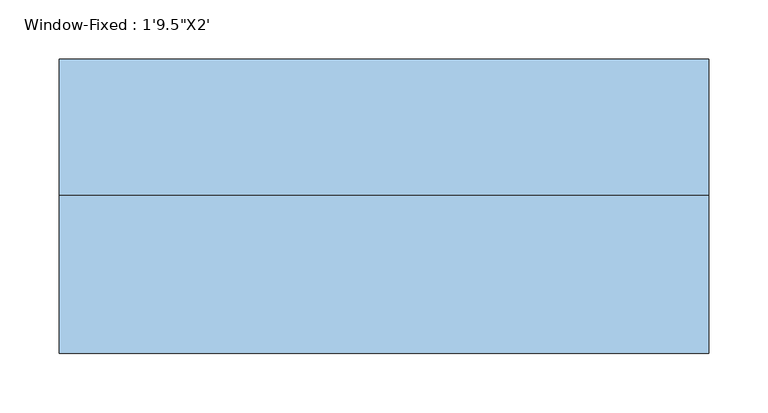
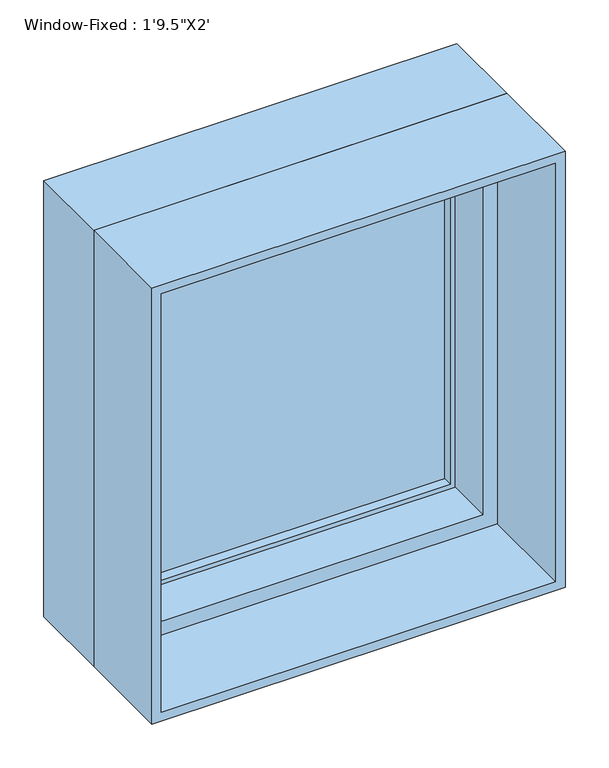
"""IFC4 building model written with IfcOpenShell, lengths in millimetres: window geometry."""

from ifc_helpers import new_model, si_unit, frame, origin, place, context, project, spatial, polyline, outline, extrude, faceted_brep, source, transform, mapped, element, save


def window_6ec6991e(model_context):
    return source(origin(), model_context, "Body", "SolidModel", [
        faceted_brep([(273.05, 19.05, 2743.2), (273.05, 133.35, 2743.2), (-273.05, 133.35, 2743.2), (-273.05, 19.05, 2743.2), (-273.05, 133.35, 2133.6), (-273.05, 19.05, 2133.6), (273.05, 133.35, 2133.6), (273.05, 19.05, 2133.6), (241.3, 19.05, 2711.45), (241.3, 19.05, 2165.35), (-241.3, 19.05, 2165.35), (-241.3, 19.05, 2711.45), (-260.35, 133.35, 2730.5), (-260.35, 133.35, 2146.3), (260.35, 133.35, 2146.3), (260.35, 133.35, 2730.5), (241.3, 82.55, 2711.45), (-241.3, 82.55, 2711.45), (260.35, 82.55, 2730.5), (-260.35, 82.55, 2730.5), (-241.3, 82.55, 2165.35), (-260.35, 82.55, 2146.3), (241.3, 82.55, 2165.35), (260.35, 82.55, 2146.3)], [[[0, 1, 2, 3]], [[3, 2, 4, 5]], [[5, 4, 6, 7]], [[3, 5, 7, 0], [8, 9, 10, 11]], [[7, 6, 1, 0]], [[1, 6, 4, 2], [12, 13, 14, 15]], [[16, 8, 11, 17]], [[15, 18, 19, 12]], [[17, 11, 10, 20]], [[12, 19, 21, 13]], [[20, 10, 9, 22]], [[13, 21, 23, 14]], [[22, 9, 8, 16]], [[18, 23, 21, 19], [17, 20, 22, 16]], [[14, 23, 18, 15]]]),
        extrude(outline(polyline([(2743.2, -273.05), (2133.6, -273.05), (2133.6, 273.05), (2743.2, 273.05), (2743.2, -273.05)]), holes=[polyline([(2730.5, 260.35), (2146.3, 260.35), (2146.3, -260.35), (2730.5, -260.35), (2730.5, 260.35)])]), frame((0.0, -114.3, 0.0), z_axis=(0.0, 1.0, 0.0), x_axis=(0.0, 0.0, 1.0)), (0.0, 0.0, 1.0), 133.35),
        extrude(outline(polyline([(2146.3, 260.35), (2730.5, 260.35), (2730.5, -260.35), (2146.3, -260.35), (2146.3, 260.35)]), holes=[polyline([(2171.7, -234.95), (2705.1, -234.95), (2705.1, 234.95), (2171.7, 234.95), (2171.7, -234.95)])]), frame((0.0, 82.55, 0.0), z_axis=(0.0, 1.0, 0.0), x_axis=(0.0, 0.0, 1.0)), (0.0, 0.0, 1.0), 44.45),
        extrude(outline(polyline([(234.95, 114.3), (234.95, 107.95), (-234.95, 107.95), (-234.95, 114.3), (234.95, 114.3)])), frame((0.0, 0.0, 2171.7), z_axis=(0.0, 0.0, 1.0), x_axis=(1.0, 0.0, 0.0)), (0.0, 0.0, 1.0), 533.4),
        extrude(outline(polyline([(-234.95, 95.25), (-234.95, 101.6), (234.95, 101.6), (234.95, 95.25), (-234.95, 95.25)])), frame((0.0, 0.0, 2171.7), z_axis=(0.0, 0.0, 1.0), x_axis=(1.0, 0.0, 0.0)), (0.0, 0.0, 1.0), 533.4),
    ])


if __name__ == "__main__":
    model = new_model("IFC4")
    model_context = context("Model", 3, world=origin())
    ifc_project = project(units=[si_unit("LENGTHUNIT", "METRE", prefix="MILLI")], contexts=[model_context])
    site = spatial("IfcSite", under=ifc_project)
    building = spatial("IfcBuilding", under=site)
    placement = place(None, origin())
    window_shape = window_6ec6991e(model_context)
    element("IfcWindow", 1, ObjectType="Window-Fixed : 1'9.5\"X2'", at=placement, inside=building, context=model_context, shape_type="MappedRepresentation", body=[
        mapped(window_shape, transform((0.0, 0.0, 0.0), x_axis=(1.0, 0.0, 0.0), y_axis=(0.0, 1.0, 0.0), z_axis=(0.0, 0.0, 1.0))),
    ])
    save(model, "model.ifc")

# Revit data of these elements
# Type "Window-Fixed : 1'9.5\"X2'"
#   Type Mark = "29"
#   Fire Rating = "0.5h"
#   Assembly Code = "B2020100"
#   Analytic Construction = "Double glazing - domestic"
#   Window Inset [instance default] = 0' - 0"
#   Wall Thickness [instance default] = 0' - 6"
#   Visual Light Transmittance = 0.81
#   Thermal Resistance (R) = 1.8146 (h·ft²·°F)/BTU
#   Solar Heat Gain Coefficient = 0.76
#   Rough Width = 1' - 10"
#   Rough Height = 2' - 0 1/2"
#   Interior Wall Closure [instance default] = 0' - 2 1/4"
#   Height = 2' - 0"
#   Heat Transfer Coefficient (U) = 0.5511 BTU/(h·ft²·°F)
#   Frame Extension [instance default] = 0' - 0 1/4"
#   Exterior Wall Closure [instance default] = 0' - 1 1/4"
#   Extension Jamb [instance default] = 0' - 2 1/4"
#   Default Sill Height = 7' - 0"
#   Width = 1' - 9 1/2"
#   Muntin Visibility = yes
#   Interior Trim Visibility [instance default] = yes
#   Exterior Trim Visibility [instance default] = yes
#   Extension Jamb Visibility [instance default] = yes
#   Muntin Pattern = Muntin Pattern_2x2 : Muntin Pattern_2x2
#   Interior Trim Material = Wood - Stained
#   Interior Trim = Trim-Window-Interior-Flat : Picture Frame
#   Interior Frame Material = Wood - Stained
#   Glass Panel Material = Glass
#   Exterior Trim Material = Clad - White
#   Exterior Trim = Trim-Window-Exterior-Flat : with Sill
#   Exterior Frame Material = Clad - White
#   Wall Closure = (empty or 0)
# Element 1 (IfcWindow, "Window-Fixed : 1'9.5\"X2'")
#   Wall Thickness = 0' - 9"
#   Extension Jamb = 0' - 5 1/4"
#   Materials on its faces: "Wood - Stained", "Glass", "Clad - White"
# Materials
#   "Wood - Stained": class "Wood", colour RGB 224 178 126, transparency 0, Cost = 0
#   "Glass": class "Glass", colour RGB 0 128 192, transparency 0.75, Description = "Soda Lime Glass", Cost = 0
#   "Clad - White": class "Wood", colour RGB 242 242 238, transparency 0, Cost = 0
